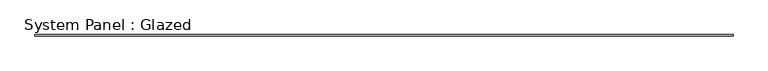
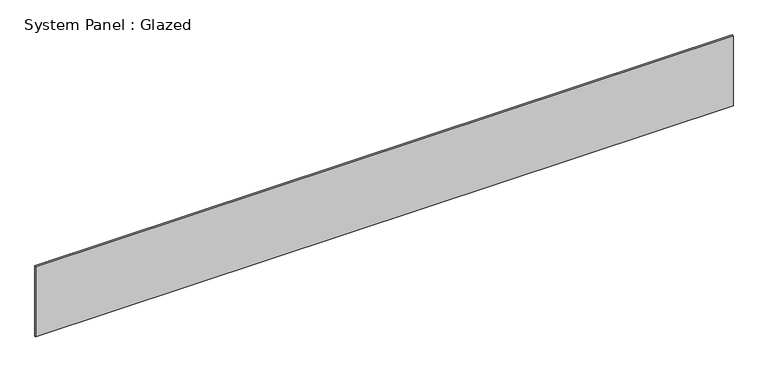
"""IFC4 building model written with IfcOpenShell, lengths in millimetres: plate geometry, System Panel : Glazed."""

from ifc_helpers import new_model, si_unit, origin, origin_with_axes, place, context, project, spatial, polyline, outline, extrude, source, transform, mapped, element, save


def system_panel_glazed_6e908680(model_context):
    return source(origin(), model_context, "Body", "SweptSolid", [
        extrude(outline(polyline([(6851.65, 19.05), (-6851.65, 19.05), (-6851.65, 44.45), (6851.65, 44.45), (6851.65, 19.05)])), origin_with_axes(), (0.0, 0.0, 1.0), 1460.5),
    ])


if __name__ == "__main__":
    model = new_model("IFC4")
    model_context = context("Model", 3, world=origin())
    ifc_project = project(units=[si_unit("LENGTHUNIT", "METRE", prefix="MILLI")], contexts=[model_context])
    site = spatial("IfcSite", under=ifc_project)
    building = spatial("IfcBuilding", under=site)
    placement = place(None, origin())
    system_panel_glazed_shape = system_panel_glazed_6e908680(model_context)
    element("IfcPlate", 1, ObjectType="System Panel : Glazed", at=placement, inside=building, context=model_context, shape_type="MappedRepresentation", body=[
        mapped(system_panel_glazed_shape, transform((0.0, 0.0, 0.0), x_axis=(1.0, 0.0, 0.0), y_axis=(0.0, 1.0, 0.0), z_axis=(0.0, 0.0, 1.0))),
    ])
    save(model, "model.ifc")

# Revit data of these elements
# Type "System Panel : Glazed"
#   Construction Type Id = "GSP4R"
#   Analytic Construction = "1/8 in Pilkington single glazing"
#   Visual Light Transmittance = 0.9
#   Solar Heat Gain Coefficient = 0.86
#   Heat Transfer Coefficient (U) = 1.18115 BTU/(h·ft²·°F)
# Element 1 (IfcPlate, "System Panel : Glazed")
#   Materials on its faces: "Glass"
# Materials
#   "Glass": class "Glass", colour RGB 0 128 192, transparency 0.75, Description = "Soda Lime Glass", Cost = 0
